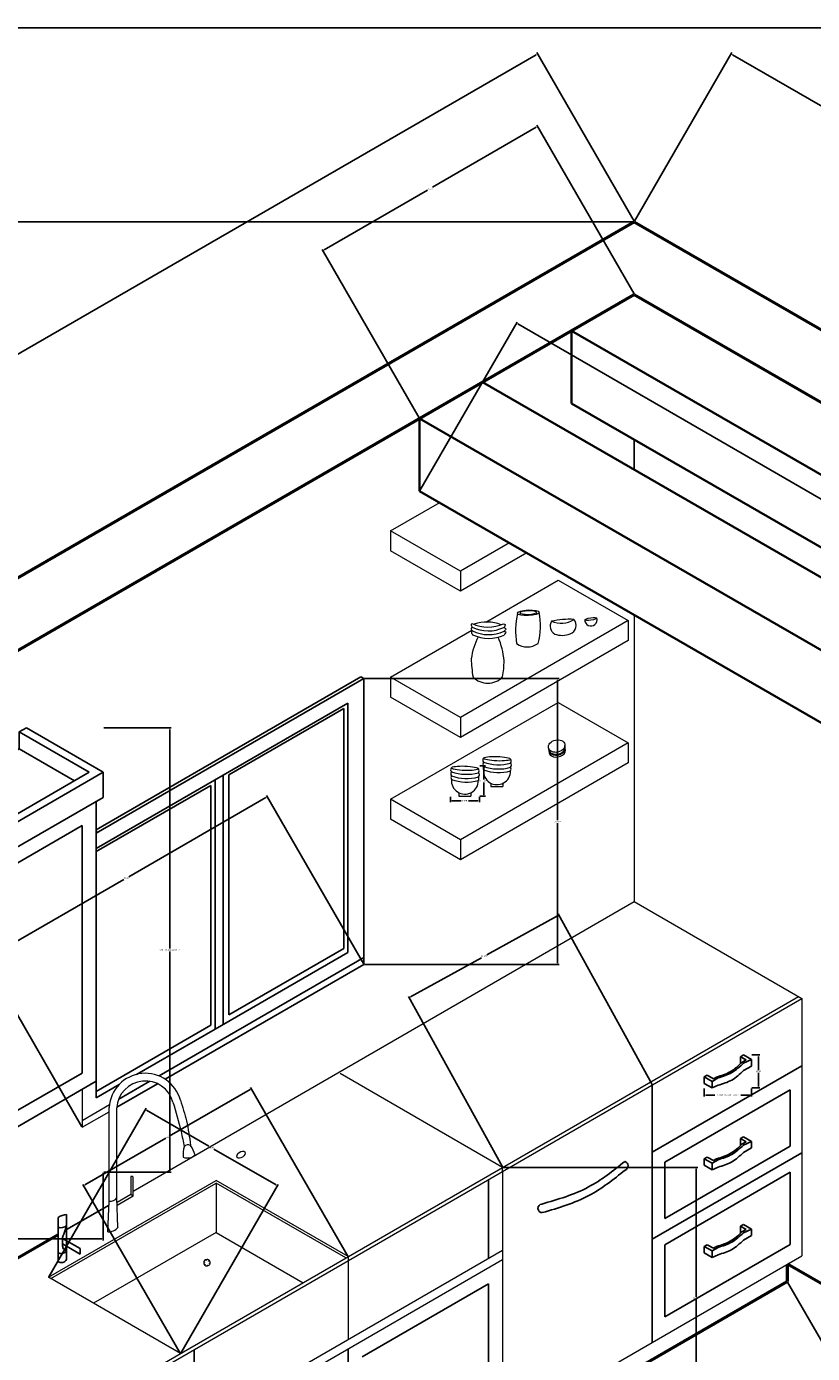
# Model space of a CAD drawing. Units: inches. Extents: x 4150 to 4636, y 2169 to 2592.
# Tile 6 of 8: x 4286 to 4383, y 2428 to 2592. Entities that reach past the tile are written whole.
import ezdxf

# ---------------------------------------------------------------- set-up
doc = ezdxf.new("R2010")
doc.units = ezdxf.units.IN
for name, color, linetype, lineweight in [('A-ANNO-DIMS', 2, 'Continuous', 18), ('A-EQPM', 6, 'Continuous', 25), ('A-FLOR-CASE', 3, 'Continuous', 25), ('A-FLOR-FIXT', 8, 'Continuous', 18), ('A-FURN', 8, 'Continuous', 18), ('A-GLAZ', 4, 'Continuous', 25), ('A-WALL', 7, 'Continuous', 50), ('S-BEAM', 1, 'Continuous', 35)]:
    doc.layers.add(name, color=color, linetype=linetype, lineweight=lineweight)
doc.styles.get("Standard").update_dxf_attribs({"font": 'arial.ttf'})
doc.dimstyles.get("Standard").update_dxf_attribs({"dimtxt": 0.18, "dimasz": 0.18, "dimexe": 0.18, "dimexo": 0.0625, "dimgap": 0.09, "dimtad": 0, "dimtih": 1, "dimtoh": 1, "dimdec": 4, "dimzin": 0, "dimdsep": 46, "dimtxsty": 'Standard', "dimcen": 0.09, "dimadec": 0, "dimazin": 0, "dimtfac": 1, "dimtdec": 4, "dimtofl": 0, "dimtmove": 0, "dimatfit": 3, "dimfxl": 1, "dimtolj": 1, "dimtzin": 0, "dimarcsym": 0})

# ---------------------------------------------------------------- blocks, each defined once
blk = doc.blocks.new('CUBOARD 1')
for p, q in [((4285.13, 2504.76), (4286, 2505.26)), ((4295.52, 2499.76), (4286, 2505.26)), ((4285.13, 2502.65), (4285.13, 2504.76)), ((4293.79, 2499.76), (4285.13, 2504.76)), ((4262.66, 2489.68), (4285.13, 2502.65)), ((4291.96, 2498.71), (4285.13, 2502.65)), ((4269.49, 2485.74), (4293.79, 2499.76)), ((4270.36, 2485.24), (4295.52, 2499.76)), ((4270.36, 2485.24), (4295.52, 2499.76)), ((4295.52, 2499.76), (4295.52, 2496.65)), ((4270.36, 2482.12), (4295.52, 2496.65)), ((4294.66, 2496.15), (4294.66, 2461.49)), ((4284.67, 2488.39), (4292.93, 2493.15)), ((4292.93, 2493.15), (4292.93, 2462.49)), ((4259.97, 2491.24), (4270.36, 2485.24)), ((4259.97, 2488.12), (4259.97, 2491.24)), ((4282.94, 2489.39), (4282.94, 2454.72)), ((4259.97, 2488.12), (4270.36, 2482.12)), ((4259.97, 2488.12), (4259.97, 2459.23)), ((4284.67, 2488.39), (4284.67, 2457.72)), ((4272.96, 2481.62), (4281.21, 2486.39)), ((4281.21, 2486.39), (4281.21, 2455.72)), ((4270.36, 2485.24), (4270.36, 2482.12)), ((4270.36, 2482.12), (4270.36, 2485.24)), ((4271.22, 2482.62), (4271.22, 2452.73)), ((4270.36, 2482.12), (4270.36, 2453.23)), ((4272.96, 2481.62), (4272.96, 2451.73)), ((4284.67, 2457.72), (4292.93, 2462.49)), ((4275.13, 2450.21), (4294.66, 2461.49)), ((4273.63, 2451.35), (4281.21, 2455.72))]:
    blk.add_line(p, q)
for centre, radius, start, end in [((4283.56, 2460.89), 0.201, 29.3135, 156.7087), ((4281.84, 2459.9), 0.201, 29.3135, 156.7087), ((4283.63, 2457.8), 0.198, 207.8897, 338.1325), ((4281.92, 2456.81), 0.198, 207.8897, 338.1325)]:
    blk.add_arc(centre, radius, start, end)
for points in [[(4283.37, 2460.97), (4283.53, 2460.79), (4283.91, 2460.36), (4283.93, 2459.31), (4283.92, 2458.33), (4283.56, 2457.83), (4283.46, 2457.7)], [(4283.73, 2460.99), (4283.89, 2460.81), (4284.27, 2460.38), (4284.29, 2459.33), (4284.28, 2458.34), (4283.91, 2457.85), (4283.82, 2457.72)], [(4281.66, 2459.98), (4281.81, 2459.8), (4282.19, 2459.37), (4282.21, 2458.32), (4282.21, 2457.34), (4281.84, 2456.84), (4281.74, 2456.71)], [(4282.02, 2460), (4282.17, 2459.82), (4282.55, 2459.39), (4282.57, 2458.34), (4282.57, 2457.35), (4282.2, 2456.86), (4282.1, 2456.73)]]:
    blk.add_open_spline(points, degree=3, knots=[0, 0, 0, 0, 0.695815, 1.679053, 3.025679, 3.502598, 3.502598, 3.502598, 3.502598])
blk = doc.blocks.new('DRAW')
for p, q in [((4374.52, 2464.53), (4374.89, 2464.74)), ((4375.22, 2464.13), (4374.52, 2464.53)), ((4374.52, 2464.53), (4374.52, 2463.67)), ((4374.69, 2463.83), (4375.22, 2464.13)), ((4374.88, 2463.72), (4375.86, 2464.18)), ((4374.89, 2464.74), (4375.86, 2464.18)), ((4375.86, 2464.18), (4375.86, 2463.37)), ((4374.88, 2462.81), (4375.86, 2463.37)), ((4370.01, 2462.03), (4370.37, 2462.24)), ((4370.98, 2461.47), (4370.01, 2462.03)), ((4370.01, 2462.03), (4370.01, 2461.22)), ((4370.98, 2460.66), (4370.01, 2461.22)), ((4370.37, 2462.24), (4371.16, 2461.79)), ((4370.98, 2461.47), (4371.73, 2461.9)), ((4370.98, 2461.47), (4370.98, 2460.66)), ((4370.98, 2460.66), (4371.73, 2460.99)), ((4371.16, 2461.79), (4371.54, 2462.01))]:
    blk.add_line(p, q)
for points in [[(4371.54, 2462.01), (4372.13, 2462.19), (4373.32, 2462.54), (4374.23, 2463.4), (4374.69, 2463.83)], [(4371.73, 2461.9), (4372.32, 2462.08), (4373.51, 2462.44), (4374.42, 2463.29), (4374.88, 2463.72)], [(4371.73, 2460.99), (4372.32, 2461.17), (4373.51, 2461.52), (4374.42, 2462.37), (4374.88, 2462.81)]]:
    blk.add_open_spline(points, degree=3, knots=[0, 0, 0, 0, 1.813605, 3.677689, 3.677689, 3.677689, 3.677689])
blk = doc.blocks.new('TAP')
for p, q in [((4296.27, 2446.62), (4296.27, 2458.25)), ((4297.22, 2447.05), (4297.22, 2458.19)), ((4298.94, 2449.67), (4298.94, 2447.44)), ((4299.25, 2447.26), (4299.25, 2449.49)), ((4296.11, 2442.82), (4296.27, 2446.62)), ((4297.35, 2443.43), (4297.22, 2447.05)), ((4298.94, 2447.44), (4297.24, 2446.46)), ((4299.25, 2447.26), (4297.25, 2446.11)), ((4299.25, 2447.26), (4298.94, 2447.44))]:
    blk.add_line(p, q)
for centre, radius, start, end in [((4300.75, 2457.98), 4.49, 14.8244, 176.5989), ((4300.75, 2457.98), 3.54, 14.8244, 176.5989), ((4308.38, 2452.45), 2.96, 161.7829, 187.4316), ((4306.07, 2452.95), 0.654, 64.0286, 140.0308), ((4302.37, 2450.91), 4.78, 17.5108, 33.3502), ((4305.95, 2453.44), 1.46, 249.9654, 311.9919), ((4299.04, 2449.49), 0.209, 1.0066, 118.9934), ((4296.42, 2447.55), 0.94, 260.71, 328.0378), ((4296.18, 2444.27), 1.45, 267.2043, 324.4974)]:
    blk.add_arc(centre, radius, start, end)
for points, knots in [([(4305.09, 2459.13), (4305.36, 2458.29), (4305.96, 2456.46), (4306.22, 2454.56), (4306.36, 2453.54)], [0, 0, 0, 0, 2.66864, 5.744321, 5.744321, 5.744321, 5.744321]), ([(4304.17, 2458.89), (4304.52, 2457.68), (4305.07, 2455.86), (4305.44, 2454), (4305.57, 2453.37)], [0, 0, 0, 0, 3.770193, 5.693413, 5.693413, 5.693413, 5.693413])]:
    blk.add_open_spline(points, degree=3, knots=knots)
blk = doc.blocks.new('*U7')
blk.add_circle((0, 0), 0.0211)
blk = doc.blocks.new('*U8')
at = {"layer": 'A-FLOR-FIXT', "color": 0, "linetype": 'ByBlock', "lineweight": -2, "transparency": 16777216}
for p, rotation in [((2236.03, 1266.07), 59.99999999999999), ((2236.12, 1265.76), 119.9999999999999), ((2236.57, 1266.23), 300), ((2236.66, 1265.92), 240), ((2236.44, 1265.68), 180)]:
    blk.add_blockref('*U7', p, dxfattribs=dict(at, rotation=rotation))
blk.add_blockref('*U7', (2236.25, 1266.3), dxfattribs=at)
blk = doc.blocks.new('CUP')
for p, q in [((1.01, 0.17), (1.01, -0.25)), ((2.48, 0.16), (2.48, -0.25)), ((1.01, -0.25), (2.48, -0.25))]:
    blk.add_line(p, q)
for centre, radius, start, end in [((0.35, 3.03), 0.352, 136.956, 223.044), ((0.5, 2.53), 0.484, 147.5288, 212.4712), ((0.45, 2.05), 0.417, 148.1892, 211.8108), ((1.95, 7.93), 5.47, 250.1795, 285.7404), ((1.95, 7.41), 5.47, 250.1795, 285.7404), ((1.76, 1.67), 1.67, 174.6384, 1.2814), ((1.95, 6.97), 5.47, 250.1795, 285.7404), ((3.17, 2.91), 0.354, 317.3223, 42.6777), ((3.21, 2.42), 0.347, 309.7221, 48.7772), ((3.12, 1.93), 0.385, 325.2266, 34.7734)]:
    blk.add_arc(centre, radius, start, end)
blk.add_ellipse((1.76, 3.21), major_axis=(-1.67, 0.06), ratio=0.166089)
blk = doc.blocks.new('*D18')
at = {"layer": 'A-ANNO-DIMS', "color": 0, "lineweight": -2, "transparency": 16777216}
for p, q in [((4370.01, 2460.6), (4370.01, 2459.6)), ((4370.19, 2459.78), (4371.34, 2459.78)), ((4375.68, 2459.78), (4374.53, 2459.78)), ((4375.86, 2460.6), (4375.86, 2459.6))]:
    blk.add_line(p, q, dxfattribs=at)
at = {"layer": 'A-ANNO-DIMS', "color": 0, "transparency": 16777216}
for points in [[(4370.19, 2459.81), (4370.19, 2459.75), (4370.01, 2459.78)], [(4375.68, 2459.81), (4375.68, 2459.75), (4375.86, 2459.78)]]:
    blk.add_solid(points, dxfattribs=at)
at = {"layer": 'Defpoints', "color": 0, "transparency": 16777216}
for p in [(4370.01, 2460.66), (4375.86, 2460.66), (4375.86, 2459.78)]:
    blk.add_point(p, dxfattribs=at)
at = {"layer": 'A-ANNO-DIMS', "color": 0, "transparency": 16777216, "insert": (4372.93, 2459.78), "char_height": 0.18, "attachment_point": 5}
blk.add_mtext('\\A1;DRAWER HANDLE 6 TYP.', dxfattribs=at)
blk = doc.blocks.new('*D19')
at = {"layer": 'A-ANNO-DIMS', "color": 0, "lineweight": -2, "transparency": 16777216}
for p, q in [((4375.92, 2464.74), (4376.92, 2464.74)), ((4376.74, 2464.56), (4376.74, 2462.88)), ((4376.74, 2460.84), (4376.74, 2462.52)), ((4375.92, 2460.66), (4376.92, 2460.66))]:
    blk.add_line(p, q, dxfattribs=at)
at = {"layer": 'A-ANNO-DIMS', "color": 0, "transparency": 16777216}
for points in [[(4376.71, 2464.56), (4376.77, 2464.56), (4376.74, 2464.74)], [(4376.71, 2460.84), (4376.77, 2460.84), (4376.74, 2460.66)]]:
    blk.add_solid(points, dxfattribs=at)
at = {"layer": 'Defpoints', "color": 0, "transparency": 16777216}
for p in [(4375.86, 2464.74), (4376.74, 2464.74), (4375.86, 2460.66)]:
    blk.add_point(p, dxfattribs=at)
at = {"layer": 'A-ANNO-DIMS', "color": 0, "transparency": 16777216, "insert": (4376.74, 2462.7), "char_height": 0.18, "attachment_point": 5}
blk.add_mtext('\\A1;4 TYP.', dxfattribs=at)
blk = doc.blocks.new('*D30')
at = {"layer": 'A-ANNO-DIMS', "color": 0, "lineweight": -2, "transparency": 16777216}
for p, q in [((4342.21, 2500.57), (4342.89, 2500.57)), ((4342.71, 2500.39), (4342.71, 2498.87)), ((4342.71, 2496.98), (4342.71, 2498.5)), ((4342.21, 2496.8), (4342.89, 2496.8))]:
    blk.add_line(p, q, dxfattribs=at)
at = {"layer": 'A-ANNO-DIMS', "color": 0, "transparency": 16777216}
for points in [[(4342.68, 2500.39), (4342.74, 2500.39), (4342.71, 2500.57)], [(4342.68, 2496.98), (4342.74, 2496.98), (4342.71, 2496.8)]]:
    blk.add_solid(points, dxfattribs=at)
at = {"layer": 'Defpoints', "color": 0, "transparency": 16777216}
for p in [(4342.14, 2500.57), (4342.71, 2500.57), (4342.14, 2496.8)]:
    blk.add_point(p, dxfattribs=at)
at = {"layer": 'A-ANNO-DIMS', "color": 0, "transparency": 16777216, "insert": (4342.71, 2498.68), "char_height": 0.18, "attachment_point": 5}
blk.add_mtext('\\A1;CUP 4 TYP.', dxfattribs=at)
blk = doc.blocks.new('*D31')
at = {"layer": 'A-ANNO-DIMS', "color": 0, "lineweight": -2, "transparency": 16777216}
for p, q in [((4338.55, 2496.73), (4338.55, 2496.05)), ((4338.73, 2496.23), (4339.89, 2496.23)), ((4341.96, 2496.23), (4340.81, 2496.23)), ((4342.14, 2496.73), (4342.14, 2496.05))]:
    blk.add_line(p, q, dxfattribs=at)
at = {"layer": 'A-ANNO-DIMS', "color": 0, "transparency": 16777216}
for points in [[(4338.73, 2496.26), (4338.73, 2496.2), (4338.55, 2496.23)], [(4341.96, 2496.26), (4341.96, 2496.2), (4342.14, 2496.23)]]:
    blk.add_solid(points, dxfattribs=at)
at = {"layer": 'Defpoints', "color": 0, "transparency": 16777216}
for p in [(4338.55, 2496.8), (4342.14, 2496.8), (4342.14, 2496.23)]:
    blk.add_point(p, dxfattribs=at)
at = {"layer": 'A-ANNO-DIMS', "color": 0, "transparency": 16777216, "insert": (4340.35, 2496.23), "char_height": 0.18, "attachment_point": 5}
blk.add_mtext('\\A1;4 TYP.', dxfattribs=at)
blk = doc.blocks.new('*D32')
at = {"layer": 'A-ANNO-DIMS', "color": 0, "lineweight": -2, "transparency": 16777216}
for p, q in [((4295.59, 2505.26), (4303.96, 2505.26)), ((4303.78, 2505.08), (4303.78, 2477.92)), ((4303.78, 2450.39), (4303.78, 2477.55)), ((4295.59, 2450.21), (4303.96, 2450.21))]:
    blk.add_line(p, q, dxfattribs=at)
at = {"layer": 'A-ANNO-DIMS', "color": 0, "transparency": 16777216}
for points in [[(4303.75, 2505.08), (4303.81, 2505.08), (4303.78, 2505.26)], [(4303.75, 2450.39), (4303.81, 2450.39), (4303.78, 2450.21)]]:
    blk.add_solid(points, dxfattribs=at)
at = {"layer": 'Defpoints', "color": 0, "transparency": 16777216}
for p in [(4295.52, 2505.26), (4303.78, 2505.26), (4295.52, 2450.21)]:
    blk.add_point(p, dxfattribs=at)
at = {"layer": 'A-ANNO-DIMS', "color": 0, "transparency": 16777216, "insert": (4303.78, 2477.74), "char_height": 0.18, "attachment_point": 5}
blk.add_mtext('\\A1;WALL CUPBOARD 1 55', dxfattribs=at)
blk = doc.blocks.new('*D33')
at = {"layer": 'A-ANNO-DIMS', "color": 0, "lineweight": -2, "transparency": 16777216}
for p, q in [((4259.97, 2450.15), (4259.97, 2441.77)), ((4295.52, 2450.15), (4295.52, 2441.77)), ((4260.15, 2441.95), (4277.53, 2441.95)), ((4295.34, 2441.95), (4277.96, 2441.95))]:
    blk.add_line(p, q, dxfattribs=at)
at = {"layer": 'A-ANNO-DIMS', "color": 0, "transparency": 16777216}
for points in [[(4260.15, 2441.98), (4260.15, 2441.92), (4259.97, 2441.95)], [(4295.34, 2441.98), (4295.34, 2441.92), (4295.52, 2441.95)]]:
    blk.add_solid(points, dxfattribs=at)
at = {"layer": 'Defpoints', "color": 0, "transparency": 16777216}
for p in [(4259.97, 2450.21), (4295.52, 2450.21), (4295.52, 2441.95)]:
    blk.add_point(p, dxfattribs=at)
at = {"layer": 'A-ANNO-DIMS', "color": 0, "transparency": 16777216, "insert": (4277.75, 2441.95), "char_height": 0.18, "attachment_point": 5}
blk.add_mtext('\\A1;36', dxfattribs=at)
blk = doc.blocks.new('*D36')
at = {"layer": 'A-ANNO-DIMS', "color": 0, "lineweight": -2, "transparency": 16777216}
for p, q in [((4174.28, 2460.03), (4174.28, 2592.15)), ((4174.46, 2591.97), (4402.51, 2591.97)), ((4631.36, 2591.97), (4403.31, 2591.97)), ((4631.54, 2412.03), (4631.54, 2592.15))]:
    blk.add_line(p, q, dxfattribs=at)
at = {"layer": 'A-ANNO-DIMS', "color": 0, "transparency": 16777216}
for points in [[(4174.46, 2592), (4174.46, 2591.94), (4174.28, 2591.97)], [(4631.36, 2592), (4631.36, 2591.94), (4631.54, 2591.97)]]:
    blk.add_solid(points, dxfattribs=at)
at = {"layer": 'Defpoints', "color": 0, "transparency": 16777216}
for p in [(4631.54, 2591.97), (4174.28, 2459.97), (4631.54, 2411.97)]:
    blk.add_point(p, dxfattribs=at)
at = {"layer": 'A-ANNO-DIMS', "color": 0, "transparency": 16777216, "insert": (4402.91, 2591.97), "char_height": 0.18, "attachment_point": 5}
blk.add_mtext('\\A1;457.3', dxfattribs=at)
blk = doc.blocks.new('*D37')
at = {"layer": 'A-ANNO-DIMS', "color": 0, "lineweight": -2, "transparency": 16777216}
for p, q in [((4361.28, 2567.97), (4150.1, 2567.97)), ((4150.28, 2567.79), (4150.28, 2379.06)), ((4150.28, 2189.96), (4150.28, 2378.69)), ((4434.34, 2189.78), (4150.1, 2189.78))]:
    blk.add_line(p, q, dxfattribs=at)
at = {"layer": 'A-ANNO-DIMS', "color": 0, "transparency": 16777216}
for points in [[(4150.25, 2567.79), (4150.31, 2567.79), (4150.28, 2567.97)], [(4150.25, 2189.96), (4150.31, 2189.96), (4150.28, 2189.78)]]:
    blk.add_solid(points, dxfattribs=at)
at = {"layer": 'Defpoints', "color": 0, "transparency": 16777216}
for p in [(4361.34, 2567.97), (4150.28, 2189.78), (4434.4, 2189.78)]:
    blk.add_point(p, dxfattribs=at)
at = {"layer": 'A-ANNO-DIMS', "color": 0, "transparency": 16777216, "insert": (4150.28, 2378.87), "char_height": 0.18, "attachment_point": 5}
blk.add_mtext('\\A1;378.2', dxfattribs=at)
blk = doc.blocks.new('*D42')
at = {"layer": 'A-ANNO-DIMS', "color": 0, "lineweight": -2, "transparency": 16777216}
for p, q in [((4349.19, 2588.66), (4256.1, 2534.92)), ((4361.31, 2568.02), (4349.25, 2588.91)), ((4162.44, 2480.84), (4255.52, 2534.58)), ((4174.25, 2460.02), (4162.19, 2480.91))]:
    blk.add_line(p, q, dxfattribs=at)
at = {"layer": 'A-ANNO-DIMS', "color": 0, "transparency": 16777216}
for points in [[(4349.17, 2588.69), (4349.2, 2588.63), (4349.34, 2588.75)], [(4162.42, 2480.87), (4162.45, 2480.81), (4162.28, 2480.75)]]:
    blk.add_solid(points, dxfattribs=at)
at = {"layer": 'Defpoints', "color": 0, "transparency": 16777216}
for p in [(4349.34, 2588.75), (4361.34, 2567.97), (4174.28, 2459.97)]:
    blk.add_point(p, dxfattribs=at)
at = {"layer": 'A-ANNO-DIMS', "color": 0, "transparency": 16777216, "insert": (4255.81, 2534.75), "char_height": 0.18, "attachment_point": 5}
blk.add_mtext('\\A1;216', dxfattribs=at)
blk = doc.blocks.new('*D43')
at = {"layer": 'A-ANNO-DIMS', "color": 0, "lineweight": -2, "transparency": 16777216}
for p, q in [((4361.37, 2568.02), (4373.43, 2588.91)), ((4373.5, 2588.66), (4504.26, 2513.17)), ((4635.59, 2437.34), (4504.83, 2512.83)), ((4623.78, 2416.52), (4635.84, 2437.41))]:
    blk.add_line(p, q, dxfattribs=at)
at = {"layer": 'A-ANNO-DIMS', "color": 0, "transparency": 16777216}
for points in [[(4373.51, 2588.69), (4373.48, 2588.63), (4373.34, 2588.75)], [(4635.61, 2437.37), (4635.58, 2437.31), (4635.75, 2437.25)]]:
    blk.add_solid(points, dxfattribs=at)
at = {"layer": 'Defpoints', "color": 0, "transparency": 16777216}
for p in [(4361.34, 2567.97), (4635.75, 2437.25), (4623.75, 2416.47)]:
    blk.add_point(p, dxfattribs=at)
at = {"layer": 'A-ANNO-DIMS', "color": 0, "transparency": 16777216, "insert": (4504.54, 2513), "char_height": 0.18, "attachment_point": 5}
blk.add_mtext('\\A1;303', dxfattribs=at)
blk = doc.blocks.new('*D45')
at = {"layer": 'A-ANNO-DIMS', "color": 0, "lineweight": -2, "transparency": 16777216}
for p, q in [((4334.77, 2534.66), (4346.83, 2555.54)), ((4346.89, 2555.3), (4403.61, 2522.55)), ((4460.9, 2489.48), (4404.17, 2522.23)), ((4449.08, 2468.66), (4461.14, 2489.54))]:
    blk.add_line(p, q, dxfattribs=at)
at = {"layer": 'A-ANNO-DIMS', "color": 0, "transparency": 16777216}
for points in [[(4346.91, 2555.32), (4346.88, 2555.27), (4346.74, 2555.39)], [(4460.91, 2489.5), (4460.88, 2489.45), (4461.05, 2489.39)]]:
    blk.add_solid(points, dxfattribs=at)
at = {"layer": 'Defpoints', "color": 0, "transparency": 16777216}
for p in [(4334.74, 2534.6), (4461.05, 2489.39), (4449.05, 2468.6)]:
    blk.add_point(p, dxfattribs=at)
at = {"layer": 'A-ANNO-DIMS', "color": 0, "transparency": 16777216, "insert": (4403.89, 2522.39), "char_height": 0.18, "attachment_point": 5}
blk.add_mtext('\\A1;132', dxfattribs=at)
blk = doc.blocks.new('*D48')
at = {"layer": 'A-ANNO-DIMS', "color": 0, "lineweight": -2, "transparency": 16777216}
for p, q in [((4349.19, 2579.66), (4336.35, 2572.25)), ((4361.31, 2559.02), (4349.25, 2579.91)), ((4322.89, 2564.48), (4335.72, 2571.89)), ((4334.7, 2543.66), (4322.65, 2564.54))]:
    blk.add_line(p, q, dxfattribs=at)
at = {"layer": 'A-ANNO-DIMS', "color": 0, "transparency": 16777216}
for points in [[(4349.17, 2579.69), (4349.2, 2579.63), (4349.34, 2579.75)], [(4322.88, 2564.5), (4322.91, 2564.45), (4322.74, 2564.39)]]:
    blk.add_solid(points, dxfattribs=at)
at = {"layer": 'Defpoints', "color": 0, "transparency": 16777216}
for p in [(4349.34, 2579.75), (4361.34, 2558.97), (4334.74, 2543.6)]:
    blk.add_point(p, dxfattribs=at)
at = {"layer": 'A-ANNO-DIMS', "color": 0, "transparency": 16777216, "insert": (4336.04, 2572.07), "char_height": 0.18, "attachment_point": 5}
blk.add_mtext('\\A1;30.72', dxfattribs=at)
blk = doc.blocks.new('*D53')
at = {"layer": 'A-ANNO-DIMS', "color": 0, "lineweight": -2, "transparency": 16777216}
for p, q in [((4315.69, 2496.64), (4298.7, 2486.83)), ((4327.81, 2476), (4315.75, 2496.89)), ((4281.08, 2476.66), (4298.07, 2486.47)), ((4292.89, 2455.84), (4280.84, 2476.73))]:
    blk.add_line(p, q, dxfattribs=at)
at = {"layer": 'A-ANNO-DIMS', "color": 0, "transparency": 16777216}
for points in [[(4315.67, 2496.67), (4315.7, 2496.61), (4315.84, 2496.73)], [(4281.07, 2476.69), (4281.1, 2476.64), (4280.93, 2476.57)]]:
    blk.add_solid(points, dxfattribs=at)
at = {"layer": 'Defpoints', "color": 0, "transparency": 16777216}
for p in [(4315.84, 2496.73), (4327.84, 2475.95), (4292.93, 2455.79)]:
    blk.add_point(p, dxfattribs=at)
at = {"layer": 'A-ANNO-DIMS', "color": 0, "transparency": 16777216, "insert": (4298.38, 2486.65), "char_height": 0.18, "attachment_point": 5}
blk.add_mtext('\\A1;40.32', dxfattribs=at)
blk = doc.blocks.new('*D54')
at = {"layer": 'A-ANNO-DIMS', "color": 0, "lineweight": -2, "transparency": 16777216}
for p, q in [((4327.9, 2511.36), (4352.02, 2511.36)), ((4351.84, 2511.18), (4351.84, 2493.83)), ((4351.84, 2476.13), (4351.84, 2493.47)), ((4327.9, 2475.95), (4352.02, 2475.95))]:
    blk.add_line(p, q, dxfattribs=at)
at = {"layer": 'A-ANNO-DIMS', "color": 0, "transparency": 16777216}
for points in [[(4351.81, 2511.18), (4351.87, 2511.18), (4351.84, 2511.36)], [(4351.81, 2476.13), (4351.87, 2476.13), (4351.84, 2475.95)]]:
    blk.add_solid(points, dxfattribs=at)
at = {"layer": 'Defpoints', "color": 0, "transparency": 16777216}
for p in [(4327.84, 2511.36), (4327.84, 2475.95), (4351.84, 2475.95)]:
    blk.add_point(p, dxfattribs=at)
at = {"layer": 'A-ANNO-DIMS', "color": 0, "transparency": 16777216, "insert": (4351.84, 2493.65), "char_height": 0.18, "attachment_point": 5}
blk.add_mtext('\\A1;35.414', dxfattribs=at)
blk = doc.blocks.new('*D55')
at = {"layer": 'A-ANNO-DIMS', "color": 0, "lineweight": -2, "transparency": 16777216}
for p, q in [((4380.31, 2436.61), (4392.37, 2415.73)), ((4392.12, 2415.79), (4308.21, 2367.35)), ((4223.67, 2318.54), (4307.58, 2366.99)), ((4211.55, 2339.18), (4223.61, 2318.3))]:
    blk.add_line(p, q, dxfattribs=at)
at = {"layer": 'A-ANNO-DIMS', "color": 0, "transparency": 16777216}
for points in [[(4392.11, 2415.82), (4392.14, 2415.77), (4392.28, 2415.88)], [(4223.66, 2318.57), (4223.69, 2318.52), (4223.52, 2318.45)]]:
    blk.add_solid(points, dxfattribs=at)
at = {"layer": 'Defpoints', "color": 0, "transparency": 16777216}
for p in [(4380.28, 2436.67), (4211.52, 2339.24), (4223.52, 2318.45)]:
    blk.add_point(p, dxfattribs=at)
at = {"layer": 'A-ANNO-DIMS', "color": 0, "transparency": 16777216, "insert": (4307.9, 2367.17), "char_height": 0.18, "attachment_point": 5}
blk.add_mtext('\\A1;194.86', dxfattribs=at)
blk = doc.blocks.new('*D58')
at = {"layer": 'A-ANNO-DIMS', "color": 0, "lineweight": -2, "transparency": 16777216}
for p, q in [((4313.73, 2460.46), (4303.71, 2454.68)), ((4325.85, 2439.82), (4313.79, 2460.71)), ((4293.26, 2448.64), (4303.27, 2454.42)), ((4305.07, 2427.82), (4293.01, 2448.71))]:
    blk.add_line(p, q, dxfattribs=at)
at = {"layer": 'A-ANNO-DIMS', "color": 0, "transparency": 16777216}
for points in [[(4313.71, 2460.49), (4313.74, 2460.43), (4313.88, 2460.55)], [(4293.24, 2448.67), (4293.27, 2448.61), (4293.1, 2448.55)]]:
    blk.add_solid(points, dxfattribs=at)
at = {"layer": 'Defpoints', "color": 0, "transparency": 16777216}
for p in [(4313.88, 2460.55), (4325.88, 2439.77), (4305.1, 2427.77)]:
    blk.add_point(p, dxfattribs=at)
at = {"layer": 'A-ANNO-DIMS', "color": 0, "transparency": 16777216, "insert": (4303.49, 2454.55), "char_height": 0.18, "attachment_point": 5}
blk.add_mtext('\\A1;24', dxfattribs=at)
blk = doc.blocks.new('*D59')
at = {"layer": 'A-ANNO-DIMS', "color": 0, "lineweight": -2, "transparency": 16777216}
for p, q in [((4288.77, 2437.27), (4300.83, 2458.15)), ((4300.9, 2457.91), (4308.6, 2453.45)), ((4316.94, 2448.64), (4309.23, 2453.09)), ((4305.13, 2427.82), (4317.19, 2448.71))]:
    blk.add_line(p, q, dxfattribs=at)
at = {"layer": 'A-ANNO-DIMS', "color": 0, "transparency": 16777216}
for points in [[(4300.91, 2457.93), (4300.88, 2457.88), (4300.74, 2458)], [(4316.96, 2448.67), (4316.93, 2448.61), (4317.1, 2448.55)]]:
    blk.add_solid(points, dxfattribs=at)
at = {"layer": 'Defpoints', "color": 0, "transparency": 16777216}
for p in [(4317.1, 2448.55), (4288.74, 2437.21), (4305.1, 2427.77)]:
    blk.add_point(p, dxfattribs=at)
at = {"layer": 'A-ANNO-DIMS', "color": 0, "transparency": 16777216, "insert": (4308.92, 2453.27), "char_height": 0.18, "attachment_point": 5}
blk.add_mtext('\\A1;18.89', dxfattribs=at)
blk = doc.blocks.new('*D60')
at = {"layer": 'A-ANNO-DIMS', "color": 0, "lineweight": -2, "transparency": 16777216}
for p, q in [((4363.54, 2461.08), (4351.91, 2482.21)), ((4351.84, 2481.96), (4343.05, 2477.13)), ((4333.61, 2471.93), (4342.4, 2476.77)), ((4344.99, 2450.87), (4333.36, 2472))]:
    blk.add_line(p, q, dxfattribs=at)
at = {"layer": 'A-ANNO-DIMS', "color": 0, "transparency": 16777216}
for points in [[(4351.83, 2481.99), (4351.86, 2481.94), (4352, 2482.05)], [(4333.59, 2471.95), (4333.62, 2471.9), (4333.45, 2471.84)]]:
    blk.add_solid(points, dxfattribs=at)
at = {"layer": 'Defpoints', "color": 0, "transparency": 16777216}
for p in [(4352, 2482.05), (4363.57, 2461.03), (4345.02, 2450.81)]:
    blk.add_point(p, dxfattribs=at)
at = {"layer": 'A-ANNO-DIMS', "color": 0, "transparency": 16777216, "insert": (4342.73, 2476.95), "char_height": 0.18, "attachment_point": 5}
blk.add_mtext('\\A1;21.177', dxfattribs=at)
blk = doc.blocks.new('*D61')
at = {"layer": 'A-ANNO-DIMS', "color": 0, "lineweight": -2, "transparency": 16777216}
for p, q in [((4345.08, 2450.81), (4369.2, 2450.81)), ((4369.02, 2450.63), (4369.02, 2434.8)), ((4369.02, 2418.61), (4369.02, 2434.44)), ((4345.08, 2418.43), (4369.2, 2418.43))]:
    blk.add_line(p, q, dxfattribs=at)
at = {"layer": 'A-ANNO-DIMS', "color": 0, "transparency": 16777216}
for points in [[(4368.99, 2450.63), (4369.05, 2450.63), (4369.02, 2450.81)], [(4368.99, 2418.61), (4369.05, 2418.61), (4369.02, 2418.43)]]:
    blk.add_solid(points, dxfattribs=at)
at = {"layer": 'Defpoints', "color": 0, "transparency": 16777216}
for p in [(4345.02, 2450.81), (4345.02, 2418.43), (4369.02, 2418.43)]:
    blk.add_point(p, dxfattribs=at)
at = {"layer": 'A-ANNO-DIMS', "color": 0, "transparency": 16777216, "insert": (4369.02, 2434.62), "char_height": 0.18, "attachment_point": 5}
blk.add_mtext('\\A1;32.387', dxfattribs=at)

msp = doc.modelspace()

# ---------------------------------------------------------------- linework, layer by layer
at = {"layer": 'A-EQPM'}
msp.add_line((4363.5739, 2461.0253), (4363.5739, 2429.1386), dxfattribs=at)
for centre, radius, start, end in [((4360.0116, 2451.005), 0.5583, 290.897482, 74.825654), ((4349.9352, 2445.7392), 0.5311, 94.628244, 271.094891)]:
    msp.add_arc(centre, radius, start, end, dxfattribs=at)
for points in [[(4349.8923, 2446.2686), (4351.8856, 2446.8499), (4355.6527, 2447.9487), (4358.7155, 2450.3929), (4360.1578, 2451.5438)], [(4349.9453, 2445.2082), (4351.9386, 2445.7896), (4355.7057, 2446.8884), (4358.7685, 2449.3325), (4360.2108, 2450.4835)]]:
    msp.add_open_spline(points, degree=3, knots=[0, 0, 0, 0, 6.15908365, 11.64066884, 11.64066884, 11.64066884, 11.64066884], dxfattribs=at)
at = {"layer": 'A-FLOR-CASE'}
for p, q in [((4361.3415, 2540.9652), (4361.3415, 2537.2435)), ((4294.8599, 2492.3175), (4294.6575, 2492.4343)), ((4363.5739, 2452.6978), (4382.1261, 2463.4088)), ((4294.6575, 2461.4859), (4294.6575, 2459.4468)), ((4294.6575, 2459.4468), (4297.511, 2461.0943)), ((4297.2211, 2458.2669), (4302.2645, 2461.1787)), ((4297.4435, 2459.2485), (4301.3032, 2461.4769)), ((4365.1432, 2451.4559), (4380.6792, 2460.4256)), ((4380.6792, 2460.4256), (4380.6792, 2453.4657)), ((4363.5739, 2441.9054), (4382.1261, 2452.6165)), ((4365.1432, 2444.4959), (4380.6792, 2453.4657)), ((4365.1432, 2451.4559), (4365.1432, 2444.4959)), ((4343.2897, 2449.3142), (4343.2897, 2439.5554)), ((4365.1432, 2441.2392), (4380.6792, 2450.209)), ((4380.6792, 2450.209), (4380.6792, 2441.2741)), ((4290.9871, 2443.1173), (4296.2482, 2446.1548)), ((4289.9267, 2439.1332), (4289.9267, 2444.6202)), ((4290.9871, 2444.9807), (4290.9871, 2439.3886)), ((4292.6821, 2440.7493), (4290.477, 2442.0224)), ((4290.477, 2441.3371), (4292.6821, 2440.064)), ((4365.1432, 2432.3043), (4380.6792, 2441.2741)), ((4365.1432, 2441.2392), (4365.1432, 2432.3043)), ((4292.6821, 2440.064), (4292.6821, 2440.7493)), ((4327.6164, 2427.3519), (4343.2897, 2436.4009)), ((4343.2897, 2436.4009), (4343.2897, 2419.4275)), ((4306.805, 2428.2498), (4306.805, 2396.363)), ((4325.8844, 2428.3519), (4325.8844, 2407.3785))]:
    msp.add_line(p, q, dxfattribs=at)
for centre, radius, start, end in [((4291.2291, 2442.5288), 2.4639, 95.635821, 121.91182), ((4290.3147, 2444.1806), 0.8459, 242.696749, 322.645063), ((4290.3147, 2440.9682), 0.8459, 242.696749, 322.645063), ((4290.3331, 2439.7751), 0.7597, 237.660975, 329.416862)]:
    msp.add_arc(centre, radius, start, end, dxfattribs=at)
msp.add_open_spline([(4290.9871, 2443.6673), (4290.8908, 2443.3262), (4290.7768, 2442.9228), (4290.5777, 2442.3857), (4290.4226, 2441.9542), (4290.4868, 2441.418), (4290.4775, 2440.7865), (4290.8039, 2440.5741), (4290.9871, 2440.4549)], degree=3, knots=[0, 0, 0, 0, 1.06159051, 1.25523145, 1.72249027, 2.40782279, 2.88195076, 3.48873605, 3.48873605, 3.48873605, 3.48873605], dxfattribs=at)
at = {"layer": 'A-FLOR-FIXT'}
for p, q in [((4361.3415, 2519.2435), (4361.3415, 2483.7364)), ((4299.2523, 2447.8892), (4361.3415, 2483.7364)), ((4361.3415, 2483.7364), (4382.1261, 2471.7364)), ((4247.9421, 2394.2653), (4382.1261, 2471.7364)), ((4283.8821, 2415.5153), (4381.6931, 2471.9864)), ((4345.0218, 2450.3142), (4382.1261, 2471.7364)), ((4382.1261, 2471.7364), (4382.1261, 2439.8497)), ((4345.0218, 2450.8142), (4324.8946, 2462.4347)), ((4292.9255, 2460.4859), (4292.9255, 2456.64)), ((4292.9255, 2456.64), (4296.2994, 2458.588)), ((4292.9255, 2455.7868), (4296.2665, 2457.7158)), ((4292.9255, 2456.64), (4292.9255, 2455.7868)), ((4345.0218, 2450.3142), (4345.0218, 2450.8142)), ((4345.0218, 2450.3142), (4345.0218, 2418.4275)), ((4288.7395, 2437.2109), (4309.5241, 2449.2109)), ((4289.0291, 2437.0437), (4309.5275, 2448.8785)), ((4325.8844, 2439.7653), (4309.5241, 2449.2109)), ((4325.5982, 2439.6001), (4309.5275, 2448.8785)), ((4309.5275, 2448.8785), (4309.5275, 2442.7467)), ((4309.5275, 2442.7467), (4294.3393, 2433.9778)), ((4309.5275, 2442.7467), (4320.288, 2436.5342)), ((4306.805, 2418.4909), (4345.0218, 2440.5554)), ((4306.805, 2417.3364), (4345.0218, 2439.4009)), ((4325.8844, 2439.7653), (4325.8844, 2429.5064)), ((4345.0218, 2418.4275), (4382.1261, 2439.8497)), ((4305.0998, 2427.7653), (4288.7395, 2437.2109))]:
    msp.add_line(p, q, dxfattribs=at)
for centre, radius, start, end in [((4308.3856, 2438.9969), 0.4099, 30.615243, 200.637479), ((4308.3759, 2439.017), 0.4086, 203.755681, 27.497041)]:
    msp.add_arc(centre, radius, start, end, dxfattribs=at)
msp.add_ellipse((4312.592, 2452.3888), major_axis=(-0.4717, -0.3417), ratio=0.60897615, dxfattribs=at)
at = {"layer": 'A-FURN'}
for p, q in [((4331.1433, 2529.6578), (4337.2233, 2533.1681)), ((4339.8036, 2524.6578), (4331.1433, 2529.6578)), ((4331.1433, 2529.6578), (4331.1433, 2527.1819)), ((4345.8836, 2528.1681), (4339.8036, 2524.6578)), ((4339.8036, 2522.1819), (4331.1433, 2527.1819)), ((4348.0278, 2526.9302), (4339.8036, 2522.1819)), ((4339.8036, 2524.6578), (4339.8036, 2522.1819)), ((4342.9462, 2518.3626), (4351.9279, 2523.5482)), ((4351.9279, 2523.5482), (4360.5882, 2518.5482)), ((4360.5882, 2518.5482), (4339.8036, 2506.5482)), ((4360.5882, 2518.5482), (4360.5882, 2516.0723)), ((4331.1433, 2511.5482), (4341.2031, 2517.3562)), ((4360.5882, 2516.0723), (4339.8036, 2504.0723)), ((4339.8036, 2506.5482), (4331.1433, 2511.5482)), ((4331.1433, 2511.5482), (4331.1433, 2509.0723)), ((4339.8036, 2504.0723), (4331.1433, 2509.0723)), ((4331.1433, 2496.4114), (4351.9279, 2508.4114)), ((4351.9279, 2508.4114), (4360.5882, 2503.4114)), ((4339.8036, 2506.5482), (4339.8036, 2504.0723)), ((4360.5882, 2503.4114), (4339.8036, 2491.4114)), ((4360.5882, 2503.4114), (4360.5882, 2500.9355)), ((4360.5882, 2500.9355), (4339.8036, 2488.9355)), ((4339.8036, 2491.4114), (4331.1433, 2496.4114)), ((4331.1433, 2496.4114), (4331.1433, 2493.9355)), ((4339.8036, 2488.9355), (4331.1433, 2493.9355)), ((4339.8036, 2491.4114), (4339.8036, 2488.9355))]:
    msp.add_line(p, q, dxfattribs=at)
for centre, radius, start, end in [((4343.1014, 2513.4203), 4.9447, 69.177024, 109.121349), ((4357.0432, 2517.3007), 10.41, 168.018665, 188.777919), ((4341.9022, 2517.9112), 7.8243, 343.856963, 12.267772), ((4352.0287, 2517.8687), 1.1215, 147.557627, 241.028852), ((4353.2898, 2508.7334), 9.9841, 86.698922, 102.774493), ((4352.2647, 2521.1053), 2.8881, 245.830922, 303.642494), ((4353.0291, 2517.9703), 1.11, 289.309719, 41.165525), ((4355.9698, 2518.6525), 0.767, 179.842392, 15.111759), ((4343.2347, 2522.4008), 4.6516, 244.596826, 294.337945), ((4343.2577, 2521.9345), 4.6516, 244.596826, 294.337945), ((4343.2808, 2521.4682), 4.6516, 244.596826, 294.337945), ((4343.3038, 2521.002), 4.6516, 244.596826, 294.337945), ((4352.3951, 2519.3777), 2.6512, 249.932188, 292.183071), ((4349.3935, 2512.7343), 8.3263, 152.798986, 172.423649), ((4336.0575, 2512.8271), 9.1788, 4.729921, 23.580079), ((4348.0706, 2517.5144), 2.2313, 233.874299, 307.143493), ((4353.7425, 2513.926), 12.6029, 180.427108, 190.80303), ((4334.7483, 2513.5399), 10.4568, 349.156751, 0.241401), ((4343.1863, 2513.3483), 2.5513, 224.38178, 315.897848)]:
    msp.add_arc(centre, radius, start, end, dxfattribs=at)
for centre, major_axis, ratio in [((4348.2039, 2519.5177), (-1.3439, -0.056), 0.26314919), ((4348.2036, 2519.5536), (-1.0116, -0.0421), 0.26314919), ((4355.9578, 2518.7487), (-0.7525, -0.1038), 0.19181705), ((4351.7231, 2503.0082), (-1.0123, -0.22), 0.73888524)]:
    msp.add_ellipse(centre, major_axis=major_axis, ratio=ratio, dxfattribs=at)
for centre, start_param, end_param in [((4351.7706, 2502.6535), 5.98782692, 9.60069285), ((4351.7577, 2502.7699), 6.07371547, 9.53097177), ((4351.8052, 2502.4151), 6.07371547, 9.53097177)]:
    msp.add_ellipse(centre, major_axis=(-1.0123, -0.22), ratio=0.73888524, start_param=start_param, end_param=end_param, dxfattribs=at)
for points, knots in [([(4341.2393, 2518.199), (4341.1901, 2518.1512), (4341.0495, 2518.0147), (4341.1784, 2517.8438), (4341.2623, 2517.7327)], [0, 0, 0, 0, 0.186655927, 0.533912499, 0.533912499, 0.533912499, 0.533912499]), ([(4341.2623, 2517.7327), (4341.1963, 2517.6708), (4341.0401, 2517.5244), (4341.1955, 2517.3609), (4341.2853, 2517.2664)], [0, 0, 0, 0, 0.236271505, 0.559458232, 0.559458232, 0.559458232, 0.559458232]), ([(4341.2853, 2517.2664), (4341.2437, 2517.2397), (4341.0791, 2517.1342), (4341.2104, 2516.9429), (4341.3083, 2516.8001)], [0, 0, 0, 0, 0.136299229, 0.538193408, 0.538193408, 0.538193408, 0.538193408]), ([(4345.1517, 2518.1626), (4345.2256, 2518.1337), (4345.4425, 2518.0489), (4345.2812, 2517.8364), (4345.1747, 2517.6963)], [0, 0, 0, 0, 0.204678975, 0.600968368, 0.600968368, 0.600968368, 0.600968368]), ([(4345.1747, 2517.6963), (4345.2929, 2517.6549), (4345.5696, 2517.5579), (4345.3332, 2517.3494), (4345.1978, 2517.23)], [0, 0, 0, 0, 0.298342478, 0.698407161, 0.698407161, 0.698407161, 0.698407161]), ([(4345.1978, 2517.23), (4345.2717, 2517.2244), (4345.5252, 2517.2049), (4345.347, 2516.9467), (4345.2208, 2516.7638)], [0, 0, 0, 0, 0.188827012, 0.64737969, 0.64737969, 0.64737969, 0.64737969])]:
    msp.add_open_spline(points, degree=3, knots=knots, dxfattribs=at)
at = {"layer": 'A-GLAZ'}
for p, q in [((4294.6575, 2492.628), (4327.4718, 2511.5734)), ((4294.6575, 2492.2007), (4327.8419, 2511.3597)), ((4327.8419, 2511.3597), (4327.4718, 2511.5734)), ((4327.8419, 2511.3597), (4327.8419, 2476.799)), ((4294.6575, 2490.3197), (4325.8344, 2508.3197)), ((4311.112, 2499.4329), (4325.3444, 2507.6499)), ((4325.3444, 2507.6499), (4325.3444, 2477.9279)), ((4325.8344, 2477.4468), (4325.8344, 2508.3197)), ((4309.3799, 2498.8197), (4309.3799, 2467.9468)), ((4310.3837, 2468.5263), (4310.3837, 2499.3992)), ((4311.112, 2499.4329), (4311.112, 2469.7108)), ((4294.6575, 2489.9329), (4308.8767, 2498.1423)), ((4308.8767, 2498.1423), (4308.8767, 2468.4202)), ((4309.3799, 2467.9468), (4325.8344, 2477.4468)), ((4311.112, 2469.7108), (4325.3444, 2477.9279)), ((4302.4473, 2462.1374), (4327.8419, 2476.799)), ((4303.219, 2461.7298), (4327.8419, 2475.9458)), ((4327.8419, 2476.799), (4327.8419, 2475.9458)), ((4308.8767, 2468.4202), (4294.6575, 2460.2108)), ((4299.671, 2462.3413), (4309.3799, 2467.9468))]:
    msp.add_line(p, q, dxfattribs=at)
at = {"layer": 'A-WALL'}
for p, q in [((4278.203, 2519.9652), (4361.3415, 2567.9652)), ((4361.3415, 2567.9652), (4506.8337, 2483.9652)), ((4182.0742, 2455.4652), (4361.3415, 2558.9652)), ((4361.3415, 2558.9652), (4615.9529, 2411.9652)), ((4361.3415, 2558.9652), (4454.8722, 2504.9652)), ((4190.7345, 2385.2364), (4289.9267, 2442.5051)), ((4380.2767, 2438.782), (4380.2767, 2436.6687)), ((4384.7242, 2436.2926), (4380.3446, 2438.8212)), ((4342.7355, 2414.9942), (4380.2767, 2436.6687))]:
    msp.add_line(p, q, dxfattribs=at)
at = {"layer": 'S-BEAM'}
for p, q in [((4353.5472, 2554.4652), (4467.8626, 2488.4652)), ((4353.5472, 2554.4652), (4353.5472, 2545.4652)), ((4342.5299, 2548.1043), (4456.8453, 2482.1043)), ((4353.5472, 2545.4652), (4466.3233, 2480.3539)), ((4334.7357, 2543.6043), (4449.0511, 2477.6043)), ((4334.7357, 2543.6043), (4334.7357, 2534.6043)), ((4334.7357, 2534.6043), (4449.0511, 2468.6043))]:
    msp.add_line(p, q, dxfattribs=at)

# ---------------------------------------------------------------- block references
at = {"layer": 'A-FLOR-CASE'}
for name, p in [('CUBOARD 1', (0, 0)), ('DRAW', (0, 0)), ('DRAW', (0, -10.1386)), ('DRAW', (0, -20.9976))]:
    msp.add_blockref(name, p, dxfattribs=at)
at = {"layer": 'A-FLOR-FIXT'}
for name, p in [('TAP', (0, 0)), ('*U8', (2072.0388, 1173.003))]:
    msp.add_blockref(name, p, dxfattribs=at)
at = {"layer": 'A-FURN'}
for p in [(4338.585, 2497.049), (4342.5685, 2498.2301)]:
    msp.add_blockref('CUP', p, dxfattribs=at)

# ---------------------------------------------------------------- dimensions: what is measured, and where the dimension line sits
at = {"layer": 'A-ANNO-DIMS'}
for base, p1, p2, override, picture, middle in [((4631.5414, 2591.9652), (4174.28, 2459.9652), (4631.5414, 2411.9652), {"dimdec": 1, "dimlfac": 1, "dimrnd": 0, "dimzin": 0, "dimdsep": 46, "dimlunit": 2}, '*D36', (4402.9107, 2591.9652)), ((4295.5235, 2441.9524), (4259.9665, 2450.2105), (4295.5235, 2450.2105), {"dimdec": 0, "dimlfac": 1, "dimrnd": 0, "dimzin": 0, "dimdsep": 46, "dimlunit": 2}, '*D33', (4277.745, 2441.9524))]:
    dim = msp.add_linear_dim(base=base, p1=p1, p2=p2, dimstyle='Standard', override=override, dxfattribs=at)
    dim.commit()
    dim.dimension.update_dxf_attribs({"geometry": picture, "text_midpoint": middle})
for base, p1, p2, angle, override, picture, middle in [((4349.3415, 2588.7498), (4174.28, 2459.9652), (4361.3415, 2567.9652), 30, {"dimdec": 0, "dimlfac": 1, "dimrnd": 0, "dimzin": 0, "dimdsep": 46, "dimlunit": 2}, '*D42', (4255.8107, 2534.7498)), ((4635.7472, 2437.2498), (4361.3415, 2567.9652), (4623.7472, 2416.4652), 330, {"dimdec": 0, "dimlfac": 1, "dimrnd": 0, "dimzin": 0, "dimdsep": 46, "dimlunit": 2}, '*D43', (4504.5443, 2512.9998)), ((4349.3415, 2579.7498), (4334.7357, 2543.6043), (4361.3415, 2558.9652), 30, {"dimdec": 2, "dimlfac": 1, "dimrnd": 0, "dimzin": 0, "dimdsep": 46, "dimlunit": 2}, '*D48', (4336.0386, 2572.0694)), ((4150.28, 2189.7836), (4361.3415, 2567.9652), (4434.4021, 2189.7836), 90, {"dimdec": 1, "dimlfac": 1, "dimrnd": 0, "dimzin": 0, "dimdsep": 46, "dimlunit": 2}, '*D37', (4150.28, 2378.8744)), ((4461.0511, 2489.3889), (4334.7357, 2534.6043), (4449.0511, 2468.6043), 330, {"dimdec": 0, "dimlfac": 1, "dimrnd": 0, "dimzin": 0, "dimdsep": 46, "dimlunit": 2}, '*D45', (4403.8934, 2522.3889)), ((4351.8419, 2475.9458), (4327.8419, 2511.3597), (4327.8419, 2475.9458), 270, {"dimdec": 3, "dimlfac": 1, "dimrnd": 0, "dimzin": 0, "dimdsep": 46, "dimlunit": 2}, '*D54', (4351.8419, 2493.6528)), ((4315.8419, 2496.7305), (4292.9255, 2455.7868), (4327.8419, 2475.9458), 30, {"dimdec": 2, "dimlfac": 1, "dimrnd": 0, "dimzin": 0, "dimdsep": 46, "dimlunit": 2}, '*D53', (4298.3837, 2486.6509)), ((4352.0014, 2482.051), (4345.0218, 2450.8142), (4363.5739, 2461.0253), 28.828352, {"dimdec": 3, "dimlfac": 1, "dimrnd": 0, "dimzin": 0, "dimdsep": 46, "dimlunit": 2}, '*D60', (4342.7254, 2476.9454)), ((4313.8844, 2460.5499), (4305.0998, 2427.7653), (4325.8844, 2439.7653), 30, {"dimdec": 0, "dimlfac": 1, "dimrnd": 0, "dimzin": 0, "dimdsep": 46, "dimlunit": 2}, '*D58', (4303.4921, 2454.5499)), ((4317.0998, 2448.5499), (4288.7395, 2437.2109), (4305.0998, 2427.7653), 330, {"dimdec": 2, "dimlfac": 1, "dimrnd": 0, "dimzin": 0, "dimdsep": 46, "dimlunit": 2}, '*D59', (4308.9196, 2453.2727)), ((4369.0218, 2418.4275), (4345.0218, 2450.8142), (4345.0218, 2418.4275), 270, {"dimdec": 3, "dimlfac": 1, "dimrnd": 0, "dimzin": 0, "dimdsep": 46, "dimlunit": 2}, '*D61', (4369.0218, 2434.6209)), ((4223.5191, 2318.4518), (4380.2767, 2436.6687), (4211.5191, 2339.2364), 210, {"dimdec": 2, "dimlfac": 1, "dimrnd": 0, "dimzin": 0, "dimdsep": 46, "dimlunit": 2}, '*D55', (4307.8979, 2367.1679))]:
    dim = msp.add_linear_dim(base=base, p1=p1, p2=p2, angle=angle, dimstyle='Standard', override=override, dxfattribs=at)
    dim.commit()
    dim.dimension.update_dxf_attribs({"geometry": picture, "text_midpoint": middle})
for base, p1, p2, text, picture, middle in [((4303.7817, 2505.2646), (4295.5235, 2450.2105), (4295.5235, 2505.2646), 'WALL CUPBOARD 1 <>', '*D32', (4303.7817, 2477.7376)), ((4342.7091, 2500.5671), (4342.1436, 2496.7973), (4342.1436, 2500.5671), 'CUP <> TYP.', '*D30', (4342.7091, 2498.6822)), ((4376.7374, 2464.7448), (4375.8596, 2460.6607), (4375.8596, 2464.7448), '<> TYP.', '*D19', (4376.7374, 2462.7027))]:
    dim = msp.add_linear_dim(base=base, p1=p1, p2=p2, angle=90, text=text, dimstyle='Standard', override={"dimdec": 0, "dimlfac": 1, "dimrnd": 0, "dimzin": 0, "dimdsep": 46, "dimlunit": 2}, dxfattribs=at)
    dim.commit()
    dim.dimension.update_dxf_attribs({"geometry": picture, "text_midpoint": middle})
for base, p1, p2, text, picture, middle in [((4342.1436, 2496.2318), (4338.5535, 2496.7973), (4342.1436, 2496.7973), '<> TYP.', '*D31', (4340.3486, 2496.2318)), ((4375.8596, 2459.7828), (4370.0074, 2460.6607), (4375.8596, 2460.6607), 'DRAWER HANDLE <> TYP.', '*D18', (4372.9335, 2459.7828))]:
    dim = msp.add_linear_dim(base=base, p1=p1, p2=p2, text=text, dimstyle='Standard', override={"dimdec": 0, "dimlfac": 1, "dimrnd": 0, "dimzin": 0, "dimdsep": 46, "dimlunit": 2}, dxfattribs=at)
    dim.commit()
    dim.dimension.update_dxf_attribs({"geometry": picture, "text_midpoint": middle})

doc.saveas('drawing.dxf')
